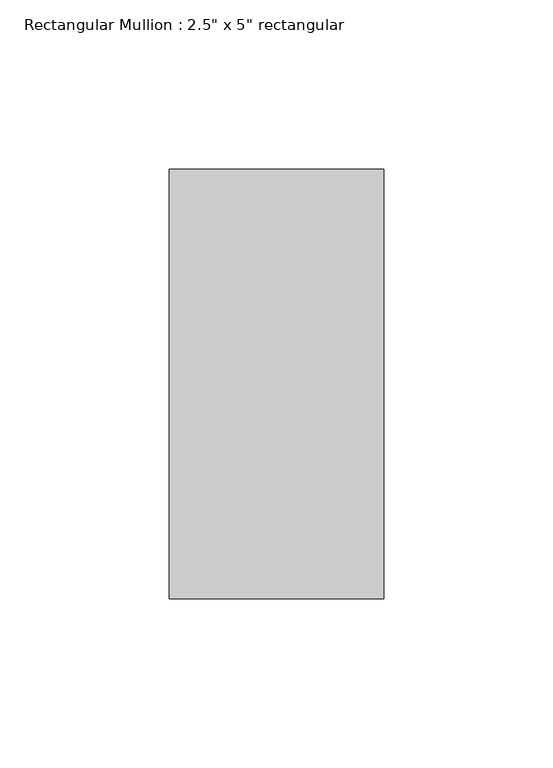
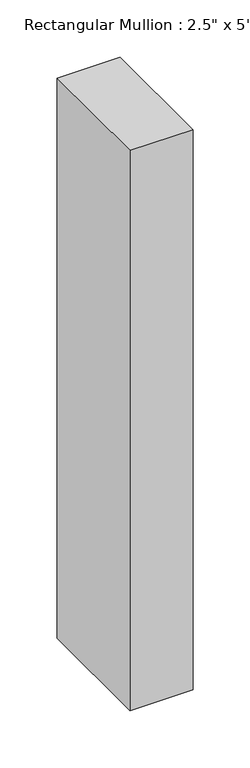
"""IFC4 building model written with IfcOpenShell, lengths in millimetres: member geometry."""

from ifc_helpers import new_model, si_unit, frame, origin, place, context, project, spatial, polyline, outline, extrude, source, transform, mapped, element, save


def member_546c81ed(model_context):
    return source(origin(), model_context, "Body", "SweptSolid", [
        extrude(outline(polyline([(0.0, 63.5), (0.0, -63.5), (-63.5, -63.5), (-63.5, 63.5), (0.0, 63.5)])), frame((0.0, 0.0, -596.9059963), z_axis=(0.0, 0.0, 1.0), x_axis=(1.0, 0.0, 0.0)), (0.0, 0.0, 1.0), 596.9059963),
    ])


if __name__ == "__main__":
    model = new_model("IFC4")
    model_context = context("Model", 3, world=origin())
    ifc_project = project(units=[si_unit("LENGTHUNIT", "METRE", prefix="MILLI")], contexts=[model_context])
    site = spatial("IfcSite", under=ifc_project)
    building = spatial("IfcBuilding", under=site)
    placement = place(None, origin())
    member_shape = member_546c81ed(model_context)
    element("IfcMember", 1, ObjectType="Rectangular Mullion : 2.5\" x 5\" rectangular", at=placement, inside=building, context=model_context, shape_type="MappedRepresentation", body=[
        mapped(member_shape, transform((0.0, 0.0, 0.0), x_axis=(1.0, 0.0, 0.0), y_axis=(0.0, 1.0, 0.0), z_axis=(0.0, 0.0, 1.0))),
    ])
    save(model, "model.ifc")

# Revit data of these elements
# Type "Rectangular Mullion : 2.5\" x 5\" rectangular"
#   built-in parameter 1007304 = 0.416667 (stored number, unit not read)
#   built-in parameter 1007301 = 0.104167 (stored number, unit not read)
#   built-in parameter 1007300 = 0.104167 (stored number, unit not read)
